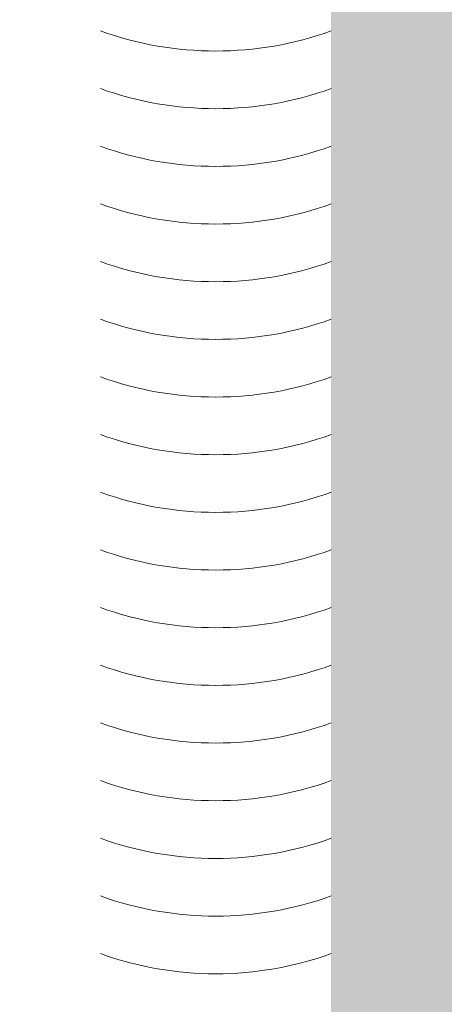
# Model space of a CAD drawing. Units: inches. Extents: x 844 to 2234, y 346 to 1084.
# Tile 13 of 93: x 1114.251 to 1116.421, y 696.22 to 701.25. Entities that reach past the tile are written whole.
import ezdxf

# ---------------------------------------------------------------- set-up
doc = ezdxf.new("R2010")
doc.units = ezdxf.units.IN
doc.header["$MEASUREMENT"] = 0
for name, color, linetype, lineweight in [('A-ANNO-DIMS', 2, 'Continuous', 18), ('furniture', 8, 'Continuous', 18), ('RA-AP-01$0$INT', 35, 'Continuous', 5)]:
    doc.layers.add(name, color=color, linetype=linetype, lineweight=lineweight)
doc.layers.add('RA-AP-01$0$FURN', color=3, linetype='Continuous')
doc.styles.get("Standard").update_dxf_attribs({"font": 'arial.ttf'})
doc.dimstyles.get("Standard").update_dxf_attribs({"dimtxt": 6, "dimasz": 3, "dimexe": 0.18, "dimexo": 0.0625, "dimgap": 0.09, "dimtad": 0, "dimtih": 1, "dimtoh": 1, "dimdec": 1, "dimzin": 0, "dimdsep": 46, "dimlunit": 3, "dimtxsty": 'Standard', "dimblk": 'ARCHTICK', "dimcen": 0.09, "dimadec": 0, "dimazin": 0, "dimtfac": 1, "dimtdec": 1, "dimtofl": 0, "dimtmove": 0, "dimatfit": 3, "dimfxl": 1, "dimtolj": 1, "dimtzin": 0, "dimarcsym": 0})

# ---------------------------------------------------------------- blocks, each defined once
blk = doc.blocks.new('A$C18D01794')
at = {"layer": 'RA-AP-01$0$INT'}
h = blk.add_hatch(color=256, dxfattribs=at)
h.paths.add_polyline_path([(4.355206456958071, -6.156712009588037), (4.355206456958071, -8.056712009588038), (5.455206456958072, -8.056712009588038), (5.455206456958072, -6.156712009588037)])
h.paths.add_polyline_path([(4.405206456958072, -8.006712009588039), (4.405206456958072, -6.206712009588038), (5.405206456958072, -6.206712009588038), (5.405206456958072, -8.006712009588039)], flags=16)
for centre in [(4.309006456955269, -7.255364458282008), (4.309006456955269, -7.278464458280756), (4.309006456953677, -7.301564458285417), (4.309006456954814, -7.324664458284166), (4.309006456954814, -7.347764458279732), (4.309006456953222, -7.37086445828462), (4.309006456955951, -7.393964458283369), (4.309006456955951, -7.417064458282117), (4.309006456954359, -7.440164458286778), (4.309006456955496, -7.463264458285527), (4.309006456955496, -7.486364458281093), (4.309006456953905, -7.509464458285981), (4.309006456952086, -7.532564458284502), (4.309006456955041, -7.555664458280295), (4.309006456954814, -7.578764458284956), (4.309006456953222, -7.601864458283705), (4.309006456951631, -7.624964458285409)]:
    blk.add_arc(centre, 0.136414042854523, 70.20384312815696, 109.7961568705686, dxfattribs=at)
blk = doc.blocks.new('A$C5D2F253E')
at = {"layer": 'RA-AP-01$0$FURN', "xscale": -0.7999999999883585, "yscale": 0.7999999999883585, "zscale": 0.8, "rotation": 90}
blk.add_blockref('A$C18D01794', (-5.687757199772477, 4.75791982714071), dxfattribs=at)
blk = doc.blocks.new('_ArchTick')
at = {"color": 0, "linetype": 'ByBlock', "const_width": 0.15}
blk.add_lwpolyline([(-0.5, -0.5), (0.5, 0.5)], dxfattribs=at)
blk = doc.blocks.new('*D144')
at = {"layer": 'A-ANNO-DIMS', "color": 0, "lineweight": -2, "transparency": 16777216}
for p, q in [((1096.615948, 439.3732739999999), (1096.615948, 1074.743301)), ((1143.115948, 492.373274), (1143.115948, 1074.743301)), ((1096.615948, 1074.563301), (1102.481950728513, 1074.563301)), ((1143.115948, 1074.563301), (1137.249945271487, 1074.563301))]:
    blk.add_line(p, q, dxfattribs=at)
at = {"layer": 'Defpoints', "color": 0, "transparency": 16777216}
for p in [(1143.115948, 1074.563301), (1143.115948, 492.3107739999999), (1096.615948, 439.3107739999999)]:
    blk.add_point(p, dxfattribs=at)
at = {"layer": 'A-ANNO-DIMS', "color": 0, "lineweight": -2, "transparency": 16777216, "xscale": 3, "yscale": 3, "zscale": 3, "rotation": 180}
blk.add_blockref('_ArchTick', (1096.615948, 1074.563301), dxfattribs=at)
at = {"layer": 'A-ANNO-DIMS', "color": 0, "lineweight": -2, "transparency": 16777216, "xscale": 3, "yscale": 3, "zscale": 3}
blk.add_blockref('_ArchTick', (1143.115948, 1074.563301), dxfattribs=at)
at = {"layer": 'A-ANNO-DIMS', "color": 0, "transparency": 16777216, "insert": (1119.865948, 1074.563301), "char_height": 6, "attachment_point": 5}
blk.add_mtext('\\A1;3\'-10 1/2"', dxfattribs=at)

msp = doc.modelspace()

# ---------------------------------------------------------------- block references
at = {"layer": 'furniture', "xscale": 15.94108302203742, "yscale": 15.94108302203742, "zscale": 15.94108302203742, "rotation": 90}
msp.add_blockref('A$C5D2F253E', (1136.147844094663, 696.2584716700112), dxfattribs=at)

# ---------------------------------------------------------------- dimensions: what is measured, and where the dimension line sits
at = {"layer": 'A-ANNO-DIMS'}
dim = msp.add_linear_dim(base=(1143.115948, 1074.563301), p1=(1096.615948, 439.3107739999999), p2=(1143.115948, 492.3107739999999), dimstyle='Standard', override={"dimdec": 1, "dimlfac": 1, "dimrnd": 0, "dimzin": 1, "dimdsep": 46, "dimlunit": 4, "dimfrac": 2}, dxfattribs=at)
dim.commit()
dim.dimension.update_dxf_attribs({"geometry": '*D144', "text_midpoint": (1119.865948, 1074.563301)})

doc.saveas('drawing.dxf')
